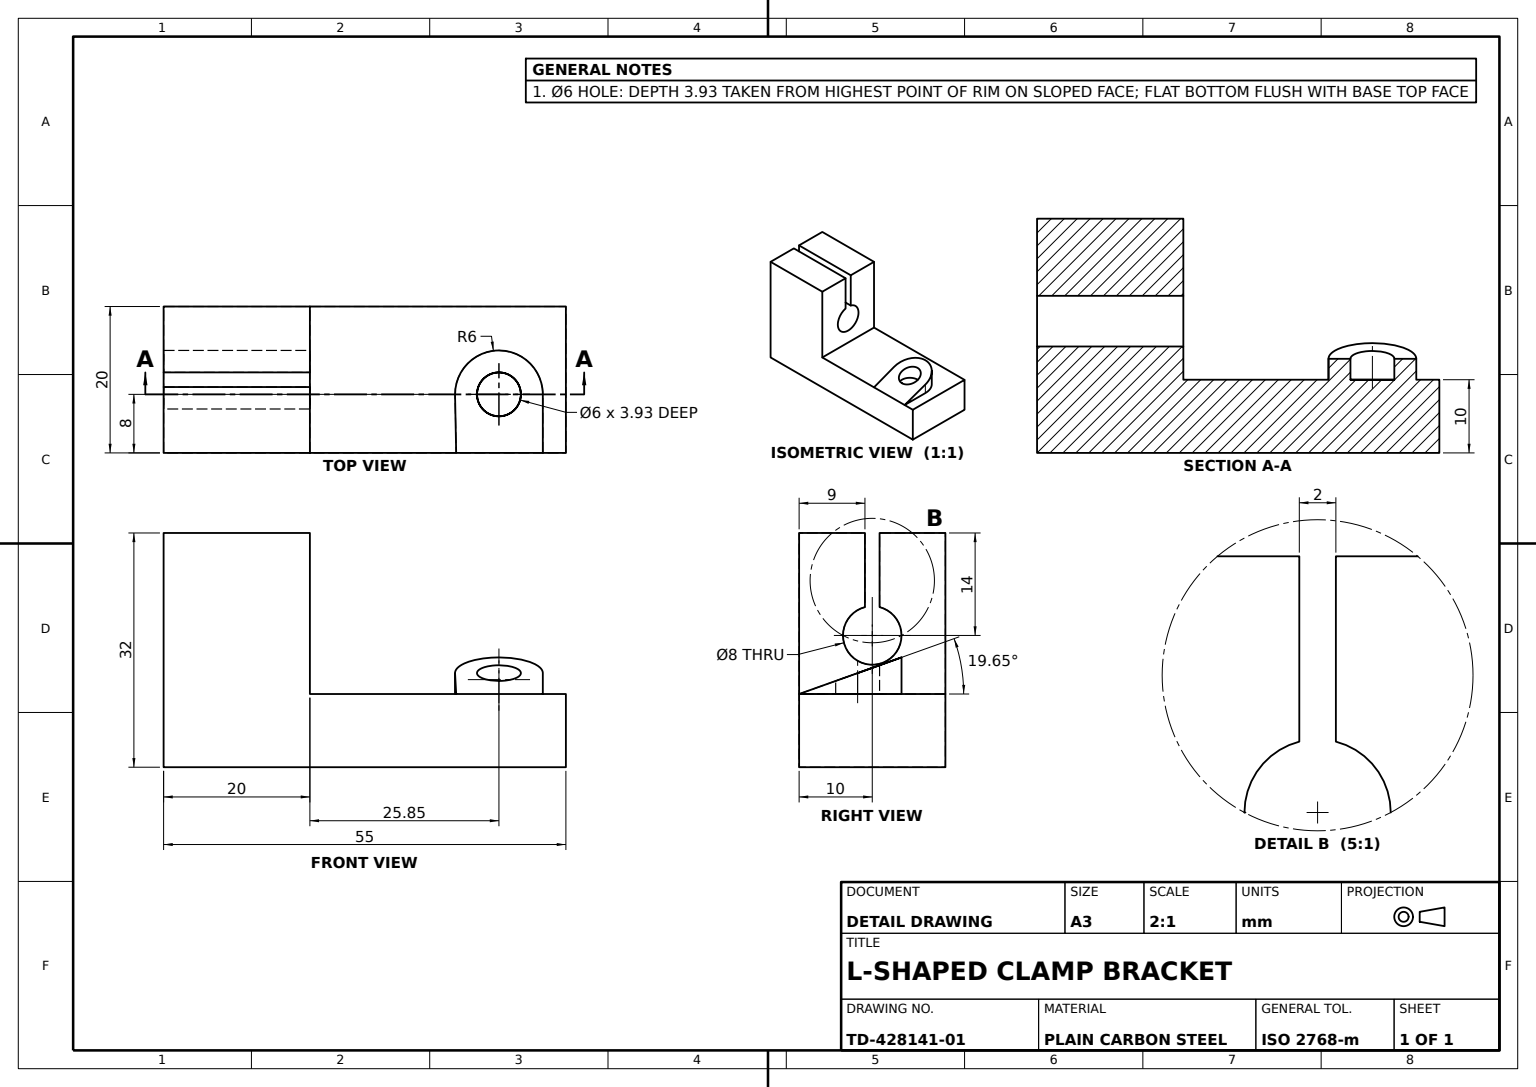
SolidWorks part; units mm, degrees
material "Plain Carbon Steel"
ref_plane "Front Plane" through (0, 0, 0) normal (0, 0, 1) x (1, 0, 0)
ref_plane "Top Plane" through (0, 0, 0) normal (0, 1, 0) x (1, 0, 0)
ref_plane "Right Plane" through (0, 0, 0) normal (1, 0, 0) x (0, 0, -1)
sketch "Bracket Profile Sketch" plane through (0, 0, 0) normal (0, 0, 1) x (1, 0, 0)
  line L6 (0, 0) -> (55, 0)
  line L7 (55, 0) -> (55, 10)
  line L8 (0, 0) -> (0, 32)
  line L9 (0, 32) -> (20, 32)
  line L10 (20, 32) -> (20, 10)
  line L11 (20, 10) -> (55, 10)
  dimension "D1" = 55
  dimension "D2" = 10
  dimension "D3" = 20
  dimension "D4" = 32
extrude "L-Bracket Body" add sketch "Bracket Profile Sketch" along normal blind 20
sketch "Clamp Bore Sketch" plane through (20, 0, 0) normal (1, 0, 0) x (0, 0, -1)
  line L0 (-20, 32) -> (0, 32) construction
  line L1 (0, 10) -> (0, 32) construction
  circle A0 centre (-10, 18) radius 4
  dimension "D1" = 8
  dimension "D2" = 14
  dimension "D3" = 10
extrude "Clamp Bore" cut sketch "Clamp Bore Sketch" against normal through all
sketch "Clamp Slit Sketch" plane through (20, 0, 0) normal (1, 0, 0) x (0, 0, -1)
  line L0 (-10, 18) -> (-10, 32.7626) construction
  line L1 (-9, 21.873) -> (-9, 32.7626)
  line L2 (-11, 21.873) -> (-11, 32.7626)
  line L3 (-11, 32.7626) -> (-9, 32.7626)
  line L5 (-11, 18) -> (-11, 32.7626) construction
  line L6 (-9, 18) -> (-9, 32.7626) construction
  line L7 (-20, 32) -> (0, 32) construction
  circle A0 centre (-10, 18) radius 4
  circle M2 centre (-10, 18) radius 4
  line M4 (0, 32) -> (-20, 32)
  dimension "D3" = 8
  dimension "D1" = 1
  dimension "D4" = 0.7626
  dimension "D5" = 10.127
  dimension "D2" = 1
extrude "Clamp Slit" cut sketch "Clamp Slit Sketch" against normal through all contours L2 L1 M2 M4
sketch "Clevis Lug Sketch" plane through (0, 10, 0) normal (0, 1, 0) x (1, 0, 0)
  line L0 (39.8472, -12.1163) -> (40, -20)
  line L1 (55, -20) -> (20, -20) construction
  line L2 (40, -20) -> (51.846, -20)
  line L3 (51.846, -20) -> (51.846, -12)
  line L4 (55, -20) -> (55, 0) construction
  line L5 (20, -20) -> (20, 0) construction
  arc A0 (51.846, -12) -> (39.8472, -12.1163) centre (45.846, -12) ccw
  circle A1 centre (45.846, -12) radius 3
  dimension "D1" = 15
  dimension "D2" = 6
  dimension "D4" = 6
  dimension "D3" = 8
  dimension "D5" = 19.8472
extrude "Clevis Lug" add sketch "Clevis Lug Sketch" along normal blind 5
sketch "Lug Pin Hole Sketch" plane through (51.846, 0, 0) normal (1, 0, 0) x (0, 0, -1)
  line L0 (-20, 15) -> (-20, 10)
  line L1 (-20, 15) -> (-20, 10) construction
  line L4 (-6, 15) -> (-20, 10)
  line L5 (-6, 15) -> (-20, 15)
  dimension "D1" = 5
extrude "Lug Pin Hole" cut sketch "Lug Pin Hole Sketch" against normal blind 12
